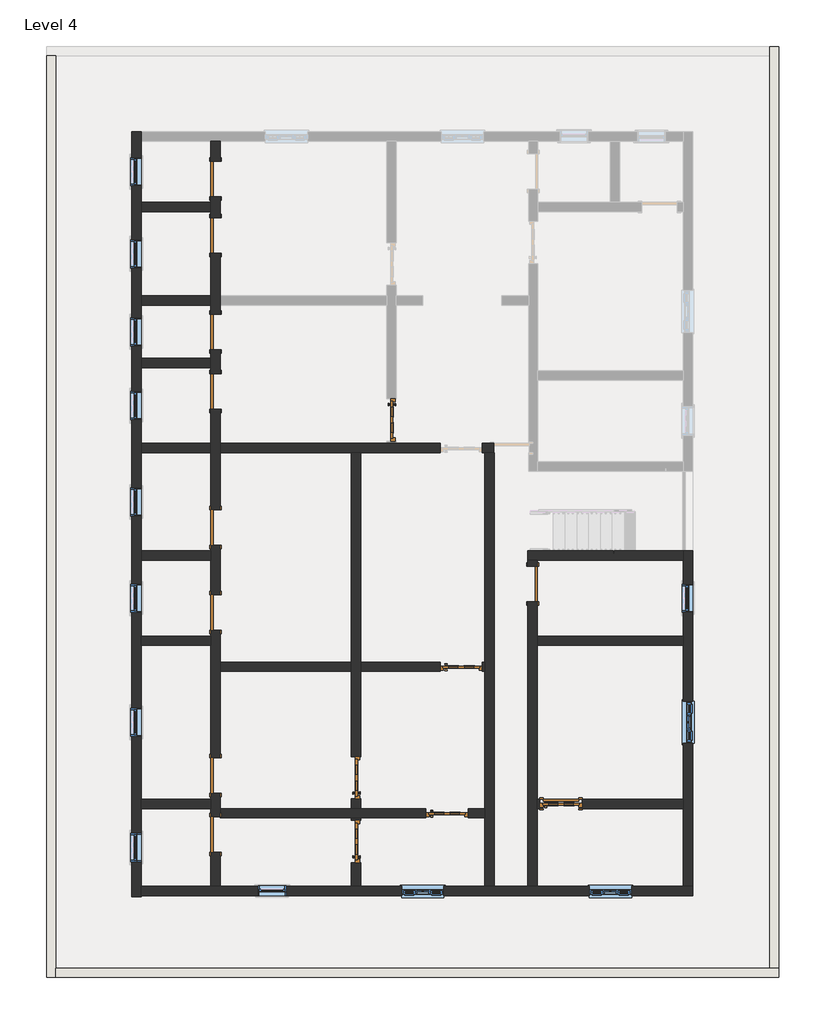
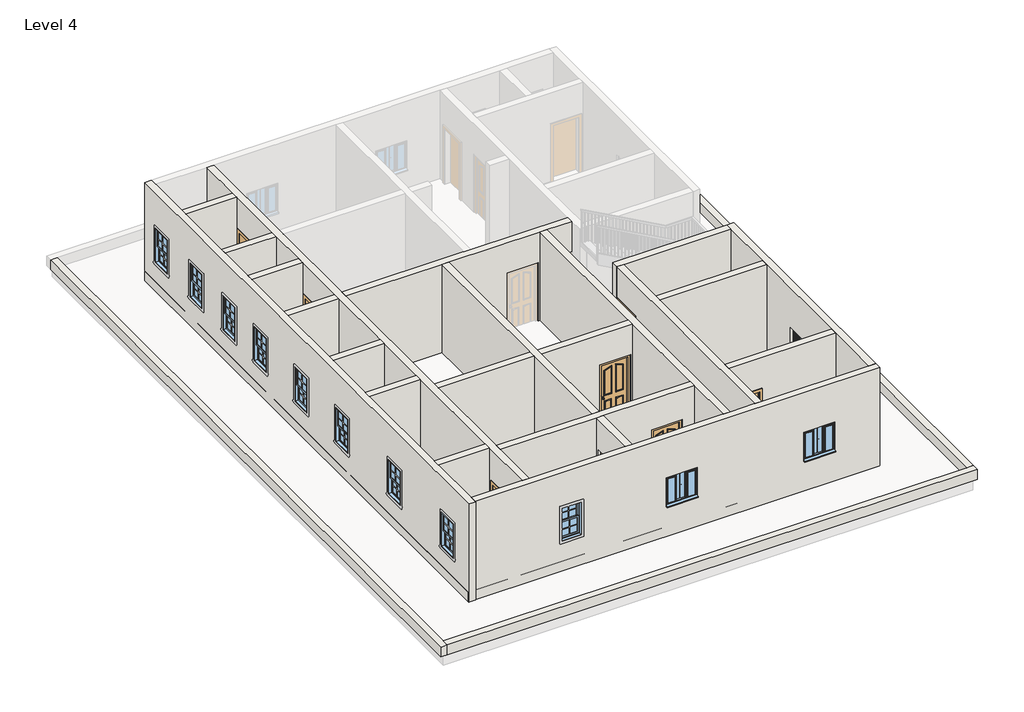
# One storey, part 1 of 3: 22 walls, 16 doors, 13 windows.
# Revit data of these elements (continued)
# Element 44 (IfcWindow, "Window-Double-Hung : 24\" x 42\"") (continued)
#   Exterior Trim Visibility = yes
#   Phase Created = New Construction
#   Materials on its faces: "Wood - Stained", "Glass", "Clad - White"
# Element 45 (IfcWindow, "Window-Double-Hung : 24\" x 42\"")
#   Mark = "67"
#   Window Inset = 0' - 0"
#   Interior Wall Closure = 0' - 1 1/2"
#   Frame Extension = 0' - 1 1/4"
#   Exterior Wall Closure = 0' - 0 1/2"
#   Interior Trim Visibility = yes
#   Indicator Visibility = yes
#   Exterior Trim Visibility = yes
#   Phase Created = New Construction
#   Materials on its faces: "Wood - Stained", "Glass", "Clad - White"
# Element 46 (IfcWindow, "Window-Double-Hung : 24\" x 42\"")
#   Mark = "68"
#   Window Inset = 0' - 0"
#   Interior Wall Closure = 0' - 1 1/2"
#   Frame Extension = 0' - 1 1/4"
#   Exterior Wall Closure = 0' - 0 1/2"
#   Interior Trim Visibility = yes
#   Indicator Visibility = yes
#   Exterior Trim Visibility = yes
#   Phase Created = New Construction
#   Materials on its faces: "Wood - Stained", "Glass", "Clad - White"
# Element 47 (IfcWindow, "Window-Double-Hung : 24\" x 42\"")
#   Mark = "69"
#   Window Inset = 0' - 0"
#   Interior Wall Closure = 0' - 1 1/2"
#   Frame Extension = 0' - 1 1/4"
#   Exterior Wall Closure = 0' - 0 1/2"
#   Interior Trim Visibility = yes
#   Indicator Visibility = yes
#   Exterior Trim Visibility = yes
#   Phase Created = New Construction
#   Materials on its faces: "Wood - Stained", "Glass", "Clad - White"
# Element 48 (IfcWindow, "Window-Double-Hung : 24\" x 42\"")
#   Mark = "70"
#   Window Inset = 0' - 0"
#   Interior Wall Closure = 0' - 1 1/2"
#   Frame Extension = 0' - 1 1/4"
#   Exterior Wall Closure = 0' - 0 1/2"
#   Interior Trim Visibility = yes
#   Indicator Visibility = yes
#   Exterior Trim Visibility = yes
#   Phase Created = New Construction
#   Materials on its faces: "Wood - Stained", "Glass", "Clad - White"
# Element 49 (IfcWindow, "Windows_Tpl_w-Glazing_Cross-Bars : 910x910mm")
#   Mark = "58"
#   Phase Created = New Construction
#   Materials on its faces: "Window Frame", "Glass"
# Element 50 (IfcWindow, "Windows_Tpl_w-Glazing_Cross-Bars : 910x910mm")
#   Mark = "75"
#   Phase Created = New Construction
#   Materials on its faces: "Window Frame", "Glass"
# Element 51 (IfcWindow, "Windows_Tpl_w-Glazing_Cross-Bars : 910x910mm")
#   Mark = "76"
#   Phase Created = New Construction
#   Materials on its faces: "Window Frame", "Glass"
# Materials
#   "Door - Glazing": colour RGB 0 0 255, transparency 0.75
#   "Door - Panel": class "Wood", colour RGB 210 159 95, transparency 0, Cost = 0
#   "Door - Frame/Mullion": class "Wood", colour RGB 212 179 113, transparency 0
#   "Door - Handle": colour RGB 246 240 166, transparency 0
#   "Door - Frame": colour RGB 118 70 51, transparency 0, Cost = 0
#   "Wood - Stained": class "Wood", colour RGB 224 178 126, transparency 0, Cost = 0
#   "Clad - White": class "Wood", colour RGB 242 242 238, transparency 0, Cost = 0
#   "Glass": class "Glass", colour RGB 0 128 192, transparency 0.75, Description = "Soda Lime Glass", Cost = 0
#   "Window Frame": colour RGB 249 249 249, transparency 0
#   "Default Wall": colour RGB 128 128 128, transparency 0, Cost = 0
#   "Tile, Porcelain, 4in": class "Generic", colour RGB 89 87 158, transparency 0, Description = "Porcelain tile, 4\", white", Cost = 0
